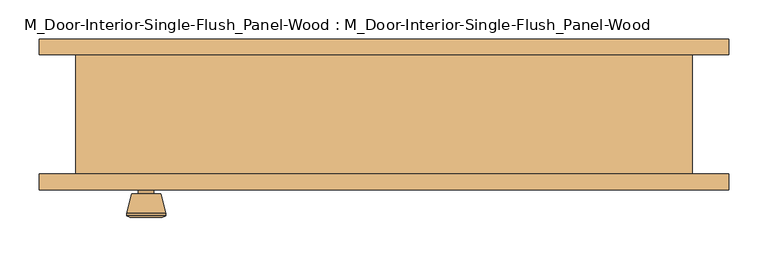
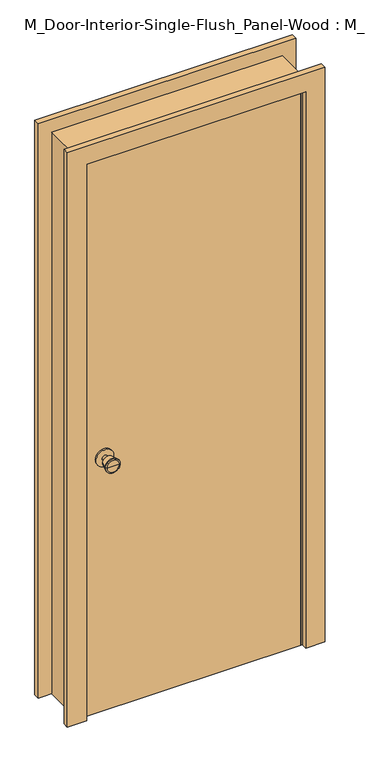
"""IFC4 building model written with IfcOpenShell, lengths in millimetres: door geometry, M_Door-Interior-Single-Flush_Panel-Wood : M_Door-Interior-Single-Flush_Panel-Wood."""

from ifc_helpers import new_model, si_unit, point, frame, frame_2d, origin, origin_with_axes, place, context, project, spatial, polyline, circle_curve, trimmed, segment, composite_curve, outline, extrude, faceted_brep, source, transform, mapped, element, save
from ifc_brep_helpers import plane_surface, cylinder_surface, revolved_surface, advanced_brep


def m_door_interior_single_flush_panel_wood_m_door_interior_b00d6502(model_context):
    return source(origin(), model_context, "Body", "SolidModel", [
        advanced_brep(
        [(-303.3, -32.025, 914.4), (-313.3, -32.025, 914.4), (-293.3, -32.025, 914.4), (-282.8241324, 16.975, 914.4), (-323.7758676, 16.975, 914.4), (-303.3, 16.975, 914.4), (-278.3, 15.1471319, 914.4), (-328.3, 15.1471319, 914.4), (-278.3, 11.6834537, 914.4), (-328.3, 11.6834537, 914.4), (-284.663764, -13.025, 914.4), (-321.936236, -13.025, 914.4), (-293.3, -13.025, 914.4), (-313.3, -13.025, 914.4)],
        [
            (0, 1),
            (1, 2, circle_curve(frame((-303.3, -32.025, 914.4), z_axis=(0.0, -1.0, 0.0), x_axis=(-1.0, 0.0, 0.0)), 10.0)),
            (2, 0),
            (2, 1, circle_curve(frame((-303.3, -32.025, 914.4), z_axis=(0.0, -1.0, 0.0), x_axis=(-1.0, 0.0, 0.0)), 10.0)),
            (3, 4, circle_curve(frame((-303.3, 16.975, 914.4), z_axis=(0.0, 1.0, 0.0), x_axis=(-1.0, 0.0, 0.0)), 20.4758676)),
            (4, 5),
            (5, 3),
            (4, 3, circle_curve(frame((-303.3, 16.975, 914.4), z_axis=(0.0, 1.0, 0.0), x_axis=(-1.0, 0.0, 0.0)), 20.4758676)),
            (6, 7, circle_curve(frame((-303.3, 15.1471319, 914.4), z_axis=(0.0, 1.0, 0.0), x_axis=(-1.0, 0.0, 0.0)), 25.0)),
            (7, 4),
            (3, 6),
            (7, 6, circle_curve(frame((-303.3, 15.1471319, 914.4), z_axis=(0.0, 1.0, 0.0), x_axis=(-1.0, 0.0, 0.0)), 25.0)),
            (8, 9, circle_curve(frame((-303.3, 11.6834537, 914.4), z_axis=(0.0, 1.0, 0.0), x_axis=(-1.0, 0.0, 0.0)), 25.0)),
            (9, 7),
            (6, 8),
            (9, 8, circle_curve(frame((-303.3, 11.6834537, 914.4), z_axis=(0.0, 1.0, 0.0), x_axis=(-1.0, 0.0, 0.0)), 25.0)),
            (10, 11, circle_curve(frame((-303.3, -13.025, 914.4), z_axis=(0.0, 1.0, 0.0), x_axis=(-1.0, 0.0, 0.0)), 18.636236)),
            (11, 9),
            (8, 10),
            (11, 10, circle_curve(frame((-303.3, -13.025, 914.4), z_axis=(0.0, 1.0, 0.0), x_axis=(-1.0, 0.0, 0.0)), 18.636236)),
            (12, 13, circle_curve(frame((-303.3, -13.025, 914.4), z_axis=(0.0, 1.0, 0.0), x_axis=(-1.0, 0.0, 0.0)), 10.0)),
            (13, 11),
            (10, 12),
            (13, 12, circle_curve(frame((-303.3, -13.025, 914.4), z_axis=(0.0, 1.0, 0.0), x_axis=(-1.0, 0.0, 0.0)), 10.0)),
            (1, 13),
            (12, 2),
        ],
        [
            plane_surface(frame((-303.3, -32.025, 914.4), z_axis=(0.0, -1.0, 0.0), x_axis=(-1.0, 0.0, 0.0))),
            plane_surface(frame((-303.3, 16.975, 914.4), z_axis=(0.0, 1.0, 0.0), x_axis=(-1.0, 0.0, 0.0))),
            revolved_surface(polyline([(-323.7758676, 16.975, 914.4), (-328.3, 15.1471319, 914.4)]), (-303.3, -32.025, 914.4), (0.0, -1.0, 0.0)),
            cylinder_surface(frame((-303.3, -32.025, 914.4), z_axis=(0.0, -1.0, 0.0), x_axis=(-1.0, 0.0, 0.0)), 25.0),
            revolved_surface(polyline([(-328.3, 11.6834537, 914.4), (-321.936236, -13.025, 914.4)]), (-303.3, -32.025, 914.4), (0.0, -1.0, 0.0)),
            plane_surface(frame((-303.3, -13.025, 914.4), z_axis=(0.0, -1.0, 0.0), x_axis=(-1.0, 0.0, 0.0))),
            cylinder_surface(frame((-303.3, -32.025, 914.4), z_axis=(0.0, -1.0, 0.0), x_axis=(-1.0, 0.0, 0.0)), 10.0),
        ],
        [
            (0, [[1, 2, 3]]),
            (0, [[-3, 4, -1]]),
            (1, [[5, 6, 7]]),
            (1, [[8, -7, -6]]),
            (2, [[9, 10, -5, 11]]),
            (2, [[12, -11, -8, -10]]),
            (3, [[13, 14, -9, 15]]),
            (3, [[16, -15, -12, -14]]),
            (4, [[17, 18, -13, 19]]),
            (4, [[20, -19, -16, -18]]),
            (5, [[21, 22, -17, 23]]),
            (5, [[24, -23, -20, -22]]),
            (6, [[-2, 25, -21, 26]]),
            (6, [[-4, -26, -24, -25]]),
        ],
    ),
        extrude(outline(composite_curve([segment(trimmed(circle_curve(frame_2d((914.4, -303.3)), 30.0), [point((914.4, -333.3))], [point((914.4, -273.3))], False, "CARTESIAN"), True, "CONTINUOUS"), segment(trimmed(circle_curve(frame_2d((914.4, -303.3)), 30.0), [point((914.4, -273.3))], [point((914.4, -333.3))], False, "CARTESIAN"), True, "CONTINUOUS")], self_intersect=False)), frame((0.0, -38.025, 0.0), z_axis=(0.0, 1.0, 0.0), x_axis=(0.0, 0.0, 1.0)), (0.0, 0.0, 1.0), 6.0),
        advanced_brep(
        [(-303.3, -79.025, 914.4), (-293.3, -79.025, 914.4), (-313.3, -79.025, 914.4), (-282.8241324, -128.025, 914.4), (-303.3, -128.025, 914.4), (-323.7758676, -128.025, 914.4), (-278.3, -126.1971319, 914.4), (-328.3, -126.1971319, 914.4), (-278.3, -122.7334537, 914.4), (-328.3, -122.7334537, 914.4), (-284.663764, -98.025, 914.4), (-321.936236, -98.025, 914.4), (-293.3, -98.025, 914.4), (-313.3, -98.025, 914.4)],
        [
            (0, 1),
            (1, 2, circle_curve(frame((-303.3, -79.025, 914.4), z_axis=(0.0, 1.0, 0.0), x_axis=(-1.0, 0.0, 0.0)), 10.0)),
            (2, 0),
            (2, 1, circle_curve(frame((-303.3, -79.025, 914.4), z_axis=(0.0, 1.0, 0.0), x_axis=(-1.0, 0.0, 0.0)), 10.0)),
            (3, 4),
            (4, 5),
            (5, 3, circle_curve(frame((-303.3, -128.025, 914.4), z_axis=(0.0, -1.0, 0.0), x_axis=(-1.0, 0.0, 0.0)), 20.4758676)),
            (3, 5, circle_curve(frame((-303.3, -128.025, 914.4), z_axis=(0.0, -1.0, 0.0), x_axis=(-1.0, 0.0, 0.0)), 20.4758676)),
            (6, 3),
            (5, 7),
            (7, 6, circle_curve(frame((-303.3, -126.1971319, 914.4), z_axis=(0.0, -1.0, 0.0), x_axis=(-1.0, 0.0, 0.0)), 25.0)),
            (6, 7, circle_curve(frame((-303.3, -126.1971319, 914.4), z_axis=(0.0, -1.0, 0.0), x_axis=(-1.0, 0.0, 0.0)), 25.0)),
            (8, 6),
            (7, 9),
            (9, 8, circle_curve(frame((-303.3, -122.7334537, 914.4), z_axis=(0.0, -1.0, 0.0), x_axis=(-1.0, 0.0, 0.0)), 25.0)),
            (8, 9, circle_curve(frame((-303.3, -122.7334537, 914.4), z_axis=(0.0, -1.0, 0.0), x_axis=(-1.0, 0.0, 0.0)), 25.0)),
            (10, 8),
            (9, 11),
            (11, 10, circle_curve(frame((-303.3, -98.025, 914.4), z_axis=(0.0, -1.0, 0.0), x_axis=(-1.0, 0.0, 0.0)), 18.636236)),
            (10, 11, circle_curve(frame((-303.3, -98.025, 914.4), z_axis=(0.0, -1.0, 0.0), x_axis=(-1.0, 0.0, 0.0)), 18.636236)),
            (12, 10),
            (11, 13),
            (13, 12, circle_curve(frame((-303.3, -98.025, 914.4), z_axis=(0.0, -1.0, 0.0), x_axis=(-1.0, 0.0, 0.0)), 10.0)),
            (12, 13, circle_curve(frame((-303.3, -98.025, 914.4), z_axis=(0.0, -1.0, 0.0), x_axis=(-1.0, 0.0, 0.0)), 10.0)),
            (1, 12),
            (13, 2),
        ],
        [
            plane_surface(frame((-303.3, -79.025, 914.4), z_axis=(0.0, 1.0, 0.0), x_axis=(-1.0, 0.0, 0.0))),
            plane_surface(frame((-303.3, -128.025, 914.4), z_axis=(0.0, -1.0, 0.0), x_axis=(-1.0, 0.0, 0.0))),
            revolved_surface(polyline([(-323.7758676, -128.025, 914.4), (-328.3, -126.1971319, 914.4)]), (-303.3, -79.025, 914.4), (0.0, 1.0, 0.0)),
            cylinder_surface(frame((-303.3, -79.025, 914.4), z_axis=(0.0, 1.0, 0.0), x_axis=(-1.0, 0.0, 0.0)), 25.0),
            revolved_surface(polyline([(-328.3, -122.7334537, 914.4), (-321.936236, -98.025, 914.4)]), (-303.3, -79.025, 914.4), (0.0, 1.0, 0.0)),
            plane_surface(frame((-303.3, -98.025, 914.4), z_axis=(0.0, 1.0, 0.0), x_axis=(-1.0, 0.0, 0.0))),
            cylinder_surface(frame((-303.3, -79.025, 914.4), z_axis=(0.0, 1.0, 0.0), x_axis=(-1.0, 0.0, 0.0)), 10.0),
        ],
        [
            (0, [[1, 2, 3]]),
            (0, [[-3, 4, -1]]),
            (1, [[5, 6, 7]]),
            (1, [[-6, -5, 8]]),
            (2, [[9, -7, 10, 11]]),
            (2, [[-10, -8, -9, 12]]),
            (3, [[13, -11, 14, 15]]),
            (3, [[-14, -12, -13, 16]]),
            (4, [[17, -15, 18, 19]]),
            (4, [[-18, -16, -17, 20]]),
            (5, [[21, -19, 22, 23]]),
            (5, [[-22, -20, -21, 24]]),
            (6, [[25, -23, 26, -2]]),
            (6, [[-26, -24, -25, -4]]),
        ],
    ),
        extrude(outline(composite_curve([segment(trimmed(circle_curve(frame_2d((914.4, -303.3)), 30.0), [point((914.4, -333.3))], [point((914.4, -273.3))], False, "CARTESIAN"), True, "CONTINUOUS"), segment(trimmed(circle_curve(frame_2d((914.4, -303.3)), 30.0), [point((914.4, -273.3))], [point((914.4, -333.3))], False, "CARTESIAN"), True, "CONTINUOUS")], self_intersect=False)), frame((0.0, -79.025, 0.0), z_axis=(0.0, 1.0, 0.0), x_axis=(0.0, 0.0, 1.0)), (0.0, 0.0, 1.0), 6.0),
        faceted_brep([(393.3, -73.025, 0.0), (368.3, -73.025, 0.0), (368.3, -38.025, 0.0), (355.6, -38.025, 0.0), (355.6, -3.1, 0.0), (368.3, -3.1, 0.0), (368.3, 79.375, 0.0), (393.3, 79.375, 0.0), (393.3, 79.375, 2025.0), (393.3, -73.025, 2025.0), (368.3, 79.375, 2000.0), (-368.3, 79.375, 2000.0), (-368.3, 79.375, 0.0), (-393.3, 79.375, 0.0), (-393.3, 79.375, 2025.0), (368.3, -3.1, 2000.0), (355.6, -3.1, 1987.3), (-355.6, -3.1, 1987.3), (-355.6, -3.1, 0.0), (-368.3, -3.1, 0.0), (-368.3, -3.1, 2000.0), (355.6, -38.025, 1987.3), (368.3, -38.025, 2000.0), (-368.3, -38.025, 2000.0), (-368.3, -38.025, 0.0), (-355.6, -38.025, 0.0), (-355.6, -38.025, 1987.3), (368.3, -73.025, 2000.0), (-393.3, -73.025, 2025.0), (-393.3, -73.025, 0.0), (-368.3, -73.025, 0.0), (-368.3, -73.025, 2000.0)], [[[0, 1, 2, 3, 4, 5, 6, 7]], [[7, 8, 9, 0]], [[6, 10, 11, 12, 13, 14, 8, 7]], [[5, 15, 10, 6]], [[4, 16, 17, 18, 19, 20, 15, 5]], [[3, 21, 16, 4]], [[2, 22, 23, 24, 25, 26, 21, 3]], [[1, 27, 22, 2]], [[0, 9, 28, 29, 30, 31, 27, 1]], [[8, 14, 28, 9]], [[15, 20, 11, 10]], [[21, 26, 17, 16]], [[27, 31, 23, 22]], [[29, 13, 12, 19, 18, 25, 24, 30]], [[14, 13, 29, 28]], [[20, 19, 12, 11]], [[26, 25, 18, 17]], [[31, 30, 24, 23]]]),
        extrude(outline(polyline([(368.3, -38.025), (368.3, -73.025), (-368.3, -73.025), (-368.3, -38.025), (368.3, -38.025)])), origin_with_axes(), (0.0, 0.0, 1.0), 2000.0),
        extrude(outline(polyline([(0.0, 439.65), (2071.35, 439.65), (2071.35, -439.65), (0.0, -439.65), (0.0, -374.65), (2006.35, -374.65), (2006.35, 374.65), (0.0, 374.65), (0.0, 439.65)])), frame((0.0, -93.025, 0.0), z_axis=(0.0, 1.0, 0.0), x_axis=(0.0, 0.0, 1.0)), (0.0, 0.0, 1.0), 20.0),
        extrude(outline(polyline([(0.0, 439.65), (2071.35, 439.65), (2071.35, -439.65), (0.0, -439.65), (0.0, -374.65), (2006.35, -374.65), (2006.35, 374.65), (0.0, 374.65), (0.0, 439.65)])), frame((0.0, 79.375, 0.0), z_axis=(0.0, 1.0, 0.0), x_axis=(0.0, 0.0, 1.0)), (0.0, 0.0, 1.0), 20.0),
    ])


if __name__ == "__main__":
    model = new_model("IFC4")
    model_context = context("Model", 3, world=origin())
    ifc_project = project(units=[si_unit("LENGTHUNIT", "METRE", prefix="MILLI")], contexts=[model_context])
    site = spatial("IfcSite", under=ifc_project)
    building = spatial("IfcBuilding", under=site)
    placement = place(None, origin())
    m_door_interior_single_flush_panel_wood_m_door_interior_shape = m_door_interior_single_flush_panel_wood_m_door_interior_b00d6502(model_context)
    element("IfcDoor", 1, ObjectType="M_Door-Interior-Single-Flush_Panel-Wood : M_Door-Interior-Single-Flush_Panel-Wood", at=placement, inside=building, context=model_context, shape_type="MappedRepresentation", body=[
        mapped(m_door_interior_single_flush_panel_wood_m_door_interior_shape, transform((0.0, 0.0, 0.0), x_axis=(1.0, 0.0, 0.0), y_axis=(0.0, 1.0, 0.0), z_axis=(0.0, 0.0, 1.0))),
    ])
    save(model, "model.ifc")

# Revit data of these elements
# Type "M_Door-Interior-Single-Flush_Panel-Wood : M_Door-Interior-Single-Flush_Panel-Wood"
#   Type Mark = "10"
#   Assembly Code = "C1020300"
#   Analytic Construction = "Wooden"
#   Thickness = 0' - 1.37795"
#   Thermal Resistance (R) = 2.5876 (h·ft²·°F)/BTU
#   Swing Angle [instance default] = 90.00°
#   Rough Width = 2' - 6.9685"
#   Rough Height = 6' - 7.72441"
#   Height = 6' - 6.74016"
#   Width = 2' - 5"
#   Heat Transfer Coefficient (U) = 0.3865 BTU/(h·ft²·°F)
#   Trim Material = Cherry
#   Panel Material = Cherry
#   Frame Material = Cherry
#   Door Handle Material = Aluminum
#   Visual Light Transmittance = 0
#   Solar Heat Gain Coefficient = 0
#   Wall Closure = (empty or 0)
#   Function = (empty or 0)
# Element 1 (IfcDoor, "M_Door-Interior-Single-Flush_Panel-Wood : M_Door-Interior-Single-Flush_Panel-Wood")
#   Materials on its faces: "Cherry", "Aluminum"
# Materials
#   "Cherry": class "Wood", colour RGB 226 177 128, transparency 0, Description = "Prunus Serotina", Cost = 0
#   "Aluminum": class "Metal", colour RGB 247 247 247, transparency 0, Description = "Aluminum 6061", Cost = 0
